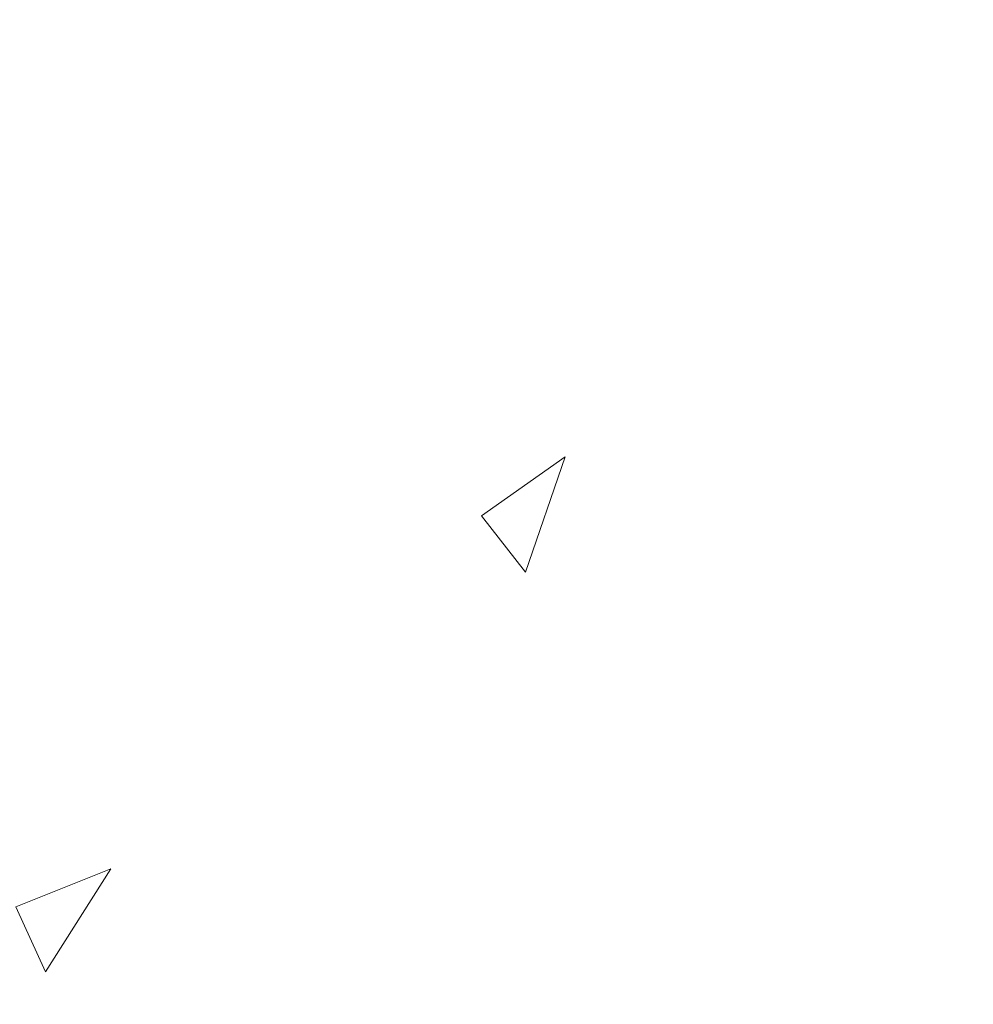
# Model space of a CAD drawing. Units: inches. Extents: x 459864 to 460310, y 324185 to 324787.
# Tile 6 of 112: x 460069.719 to 460072.714, y 324235.812 to 324238.903. Entities that reach past the tile are written whole.
import ezdxf

# ---------------------------------------------------------------- set-up
doc = ezdxf.new("R2010")
doc.units = ezdxf.units.IN
doc.layers.add('A-ANNO-DIMS', color=2, linetype='Continuous', lineweight=18)
doc.layers.add('L-HRDS', color=9, linetype='Continuous', lineweight=18)
doc.styles.get("Standard").update_dxf_attribs({"font": 'arial.ttf'})
doc.dimstyles.new('ISO-25', dxfattribs={"dimtxt": 6, "dimasz": 2.5, "dimexe": 1.25, "dimexo": 0.625, "dimtad": 1, "dimdec": 1, "dimlunit": 3, "dimtxsty": 'Standard', "dimcen": 2.5, "dimadec": 0, "dimazin": 0, "dimtfac": 1, "dimtdec": 1, "dimtmove": 0, "dimatfit": 3, "dimfxl": 1, "dimarcsym": 0})

# ---------------------------------------------------------------- blocks, each defined once
blk = doc.blocks.new('Stepping Stone - hexagonal')
for p, q in [((1.6541, 4.0806), (1.2171, 3.7716)), ((1.4471, 3.4776), (1.6541, 4.0806)), ((1.2171, 3.7716), (1.4471, 3.4776)), ((-0.7229, 1.9246), (-1.2199, 1.7256)), ((-1.0659, 1.3866), (-0.7229, 1.9246)), ((-1.2199, 1.7256), (-1.0659, 1.3866))]:
    blk.add_line(p, q)
blk = doc.blocks.new('*D37')
at = {"layer": 'A-ANNO-DIMS', "color": 0, "lineweight": -2, "transparency": 16777216}
for p, q in [((460077.6779, 324241.1222), (460077.6779, 324260.257)), ((460076.5007, 324241.1222), (460078.9279, 324241.1222)), ((460077.6779, 324231.6078), (460077.6779, 324238.6222)), ((460076.5007, 324229.1078), (460078.9279, 324229.1078))]:
    blk.add_line(p, q, dxfattribs=at)
at = {"layer": 'A-ANNO-DIMS', "color": 0, "transparency": 16777216}
for points in [[(460077.2612, 324238.6222), (460078.0946, 324238.6222), (460077.6779, 324241.1222)], [(460077.2612, 324231.6078), (460078.0946, 324231.6078), (460077.6779, 324229.1078)]]:
    blk.add_solid(points, dxfattribs=at)
at = {"layer": 'Defpoints', "color": 0, "transparency": 16777216}
for p in [(460075.8757, 324241.1222), (460077.6779, 324241.1222), (460075.8757, 324229.1078)]:
    blk.add_point(p, dxfattribs=at)
at = {"layer": 'A-ANNO-DIMS', "color": 0, "transparency": 16777216, "insert": (460073.9895, 324251.9396), "char_height": 6, "attachment_point": 5, "rotation": 90}
blk.add_mtext('1\'-0"', dxfattribs=at)

msp = doc.modelspace()

# ---------------------------------------------------------------- block references
at = {"layer": 'L-HRDS', "xscale": 0.6, "yscale": 0.6}
msp.add_blockref('Stepping Stone - hexagonal', (460070.4397, 324235.0823), dxfattribs=at)

# ---------------------------------------------------------------- dimensions: what is measured, and where the dimension line sits
at = {"layer": 'A-ANNO-DIMS'}
dim = msp.add_linear_dim(base=(460077.6779, 324241.1222), p1=(460075.8757, 324229.1078), p2=(460075.8757, 324241.1222), angle=90, dimstyle='ISO-25', override={"dimdec": 1, "dimlfac": 1, "dimrnd": 0, "dimzin": 1, "dimdsep": 46, "dimlunit": 4, "dimfrac": 2}, dxfattribs=at)
dim.commit()
dim.dimension.update_dxf_attribs({"geometry": '*D37', "text_midpoint": (460073.9895, 324251.9396)})

doc.saveas('drawing.dxf')
